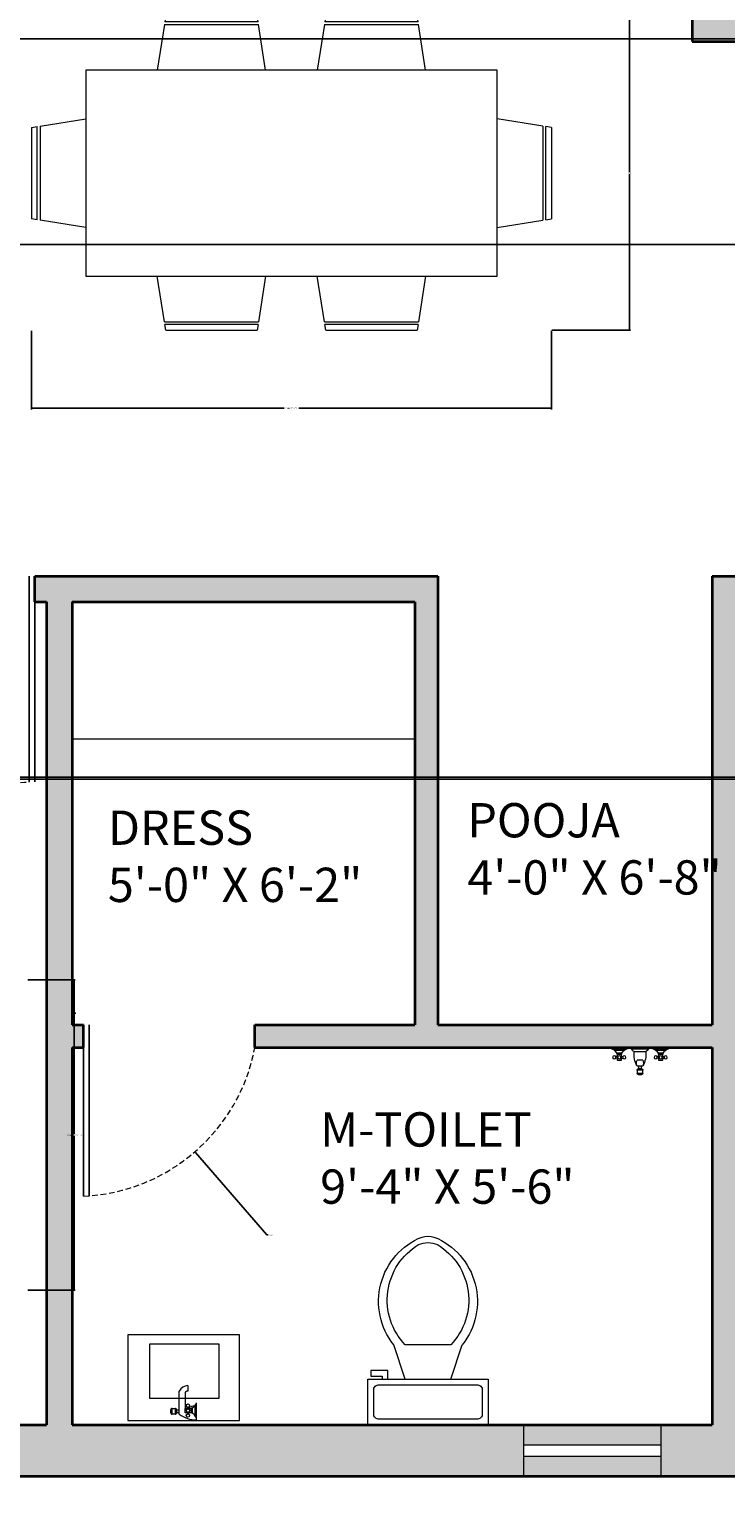
# Model space of a CAD drawing. Units: inches. Extents: x 1693 to 2974, y 2201 to 2965.
# Tile 18 of 24: x 2665 to 2787, y 2332 to 2588. Entities that reach past the tile are written whole.
import ezdxf

# ---------------------------------------------------------------- set-up
doc = ezdxf.new("R2010")
doc.units = ezdxf.units.IN
doc.header["$LTSCALE"] = 2
doc.header["$MEASUREMENT"] = 0
doc.linetypes.add('HIDDEN', pattern=[0.375, 0.25, -0.125])
for name, color, linetype, lineweight in [('A-ANNO-DIMS', 2, 'Continuous', 18), ('A-AREA-IDEN', 7, 'Continuous', 18), ('A-DOOR', 3, 'Continuous', 25), ('A-DOOR-SWNG', 3, 'HIDDEN', 13), ('A-FLOR-CASE', 32, 'Continuous', 18), ('A-FLOR-FIXT', 9, 'Continuous', 18), ('A-FURN', 8, 'Continuous', 18), ('A-GLAZ', 4, 'Continuous', 18), ('A-WALL', 7, 'Continuous', 35)]:
    doc.layers.add(name, color=color, linetype=linetype, lineweight=lineweight)
doc.layers.add('A-GLAZ-PATT', color=141, linetype='Continuous', lineweight=13, true_color=0xadddf7)
doc.layers.add('A-WALL-PATT', color=251, linetype='Continuous', lineweight=13, true_color=0x636466)
doc.styles.get("Standard").update_dxf_attribs({"font": 'arial.ttf'})
doc.dimstyles.get("Standard").update_dxf_attribs({"dimtxt": 0.18, "dimasz": 0.18, "dimexe": 0.18, "dimexo": 0.0625, "dimgap": 0.09, "dimtad": 0, "dimtih": 1, "dimtoh": 1, "dimdec": 1, "dimzin": 0, "dimdsep": 46, "dimlunit": 3, "dimtxsty": 'Standard', "dimcen": 0.09, "dimadec": 0, "dimazin": 0, "dimtfac": 1, "dimtdec": 1, "dimtofl": 0, "dimtmove": 0, "dimatfit": 3, "dimfxl": 1, "dimtolj": 1, "dimtzin": 0, "dimarcsym": 0})

# ---------------------------------------------------------------- blocks, each defined once
blk = doc.blocks.new('Toilet - top')
for p, q in [((9.5, -6), (9.5, -2)), ((-10, -8.5), (-8, -8.5)), ((-10, -9.5), (-10, -8.5)), ((-7, -9.5), (-10, -9.5)), ((-8, -8.5), (-8, -8)), ((-7, -8), (-7, -9.5)), ((-4, -8), (-6, -14)), ((4, -8), (6, -14)), ((4, -14), (-4, -14))]:
    blk.add_line(p, q)
blk.add_lwpolyline([(10.5, -8), (10.5, 0), (-10.5, 0), (-10.5, -8)], close=True)
for points in [[(-9.5, -2), (-9.5, -6)], [(8.5, -1), (-8.5, -1)], [(-8.5, -7), (8.5, -7)]]:
    blk.add_lwpolyline(points)
for centre, radius, start, end in [((-8.62, -1.88), 0.884, 81.8699, 188.1301), ((8.62, -1.88), 0.884, 351.8699, 98.1301), ((-8.62, -6.12), 0.884, 171.8699, 278.1301), ((8.62, -6.12), 0.884, 261.8699, 8.1301), ((3.52, -21.58), 12.17, 141.4691, 247.9714), ((4.2, -21.82), 11.33, 136.3677, 238.9468), ((-3.52, -21.58), 12.17, 292.0284, 38.5307), ((-4.2, -21.82), 11.33, 301.053, 43.6321), ((0, -27.88), 4, 245.7318, 294.2682), ((0, -29), 4, 254.8605, 285.1395)]:
    blk.add_arc(centre, radius, start, end)
blk = doc.blocks.new('Faucet - Bathroom side')
for p, q in [((-0.625, 4.25), (0.375, 4.25)), ((0.375, 3.75), (-0.625, 3.75)), ((-0.625, 3), (3.375, 3)), ((-0.375, 3), (-0.375, 3.5)), ((0.125, 3.5), (0.125, 3)), ((-1.625, 0), (-1.375, 0)), ((-1.375, 0), (1.375, 0)), ((-0.88366, 0.25), (0.88424, 0.25)), ((-0.375, 1.625), (-0.625, 1.625)), ((-0.375, 1.375), (-0.625, 1.375)), ((0.48078, 0.75), (-0.47286, 0.75)), ((2.875, 2), (0.375, 2)), ((0.375, 1.625), (0.625, 1.625)), ((0.375, 1.375), (0.625, 1.375)), ((4.375, 1.5), (3.375, 1.5))]:
    blk.add_line(p, q)
for points in [[(-0.625, 3.75), (-0.625, 4.25)], [(-0.375, 4.5), (0.125, 4.5)], [(0.125, 3.5), (-0.375, 3.5)], [(0.375, 4.25), (0.375, 3.75)]]:
    blk.add_lwpolyline(points)
blk.add_lwpolyline([(-0.375, 1), (-0.375, 2), (0.375, 2), (0.375, 1)], close=True)
for centre in [(-0.875, 1.5), (0, 1.5), (0.875, 1.5)]:
    blk.add_circle(centre, 0.27951)
for centre, radius, start, end in [((3.45929, -0.0281), 5.08436, 143.4467, 179.6834), ((-0.38253, 4.2575), 0.24259, 88.22243, 181.7776), ((-0.38253, 3.7424), 0.24259, 178.2224, 271.7776), ((0.13252, 4.2575), 0.24259, 358.2224, 91.77757), ((0.13252, 3.7424), 0.24259, 268.2224, 1.777565), ((2.70708, 1.4714), 1.66816, 0.9827695, 66.39737), ((-1.75, 1.375), 1.42522, 285.2551, 344.7449), ((1.75, 1.375), 1.42522, 195.2551, 254.7449), ((-2.49562, -0.286), 3.38273, 9.709485, 29.48735), ((2.96867, 1.5936), 0.41699, 347.0192, 102.9808)]:
    blk.add_arc(centre, radius, start, end)
blk = doc.blocks.new('Faucet - Bathroom front')
for p, q in [((-0.5, 4.25), (0.5, 4.25)), ((0.5, 3.75), (-0.5, 3.75)), ((-0.5, 3), (0.5, 3)), ((-0.25, 3), (-0.25, 3.5)), ((0.25, 3.5), (0.25, 3)), ((-5, 0), (-2.25, 0)), ((-4.5087, 0.25), (-2.7408, 0.25)), ((-4, 1.625), (-4.25, 1.625)), ((-4, 1.375), (-4.25, 1.375)), ((-3.1442, 0.75), (-4.0979, 0.75)), ((-3.25, 1.625), (-3, 1.625)), ((-3.25, 1.375), (-3, 1.375)), ((-1.5, 0), (1.5, 0)), ((-1, 0.5), (1, 0.5)), ((0.5, 2), (-0.5, 2)), ((2.25, 0), (5, 0)), ((2.7413, 0.25), (4.5092, 0.25)), ((3.25, 1.625), (3, 1.625)), ((3.25, 1.375), (3, 1.375)), ((4.1058, 0.75), (3.1521, 0.75)), ((4, 1.625), (4.25, 1.625)), ((4, 1.375), (4.25, 1.375))]:
    blk.add_line(p, q)
for points in [[(-0.5, 3.75), (-0.5, 4.25)], [(-0.25, 4.5), (0.25, 4.5)], [(0.25, 3.5), (-0.25, 3.5)], [(0.5, 4.25), (0.5, 3.75)]]:
    blk.add_lwpolyline(points)
for points in [[(-4, 1), (-4, 2), (-3.25, 2), (-3.25, 1)], [(3.25, 1), (3.25, 2), (4, 2), (4, 1)]]:
    blk.add_lwpolyline(points, close=True)
for centre in [(-4.5, 1.5), (-3.625, 1.5), (-2.75, 1.5), (2.75, 1.5), (3.625, 1.5), (4.5, 1.5)]:
    blk.add_circle(centre, 0.2795)
for centre, radius, start, end in [((3, 1), 4.0311, 150.2551, 187.125), ((0.6413, 2.5), 1.246, 156.3417, 203.6583), ((-0.2575, 4.2575), 0.2426, 88.22243, 181.7776), ((-0.2575, 3.7425), 0.2426, 178.2224, 271.7776), ((0.2575, 4.2575), 0.2426, 358.2224, 91.77757), ((0.2575, 3.7425), 0.2426, 268.2224, 1.777565), ((-3, 1), 4.0311, 352.875, 29.74488), ((-0.6413, 2.5), 1.246, 336.3417, 23.65835), ((-5.375, 1.375), 1.4252, 285.2551, 344.7449), ((-1.875, 1.375), 1.4252, 195.2551, 254.7449), ((-0.7962, -0.2038), 0.7327, 106.1502, 163.8498), ((0.7962, -0.2038), 0.7327, 16.1502, 73.84979), ((1.875, 1.375), 1.4252, 285.2551, 344.7449), ((5.375, 1.375), 1.4252, 195.2551, 254.7449)]:
    blk.add_arc(centre, radius, start, end)
blk = doc.blocks.new('DINING-SET-72x36-6-SEAT')
for p, q in [((23.5, 55), (23.34, 54)), ((39.66, 54), (23.35, 54)), ((23.5, 55), (39.5, 55)), ((39.66, 54), (39.5, 55)), ((51.5, 55), (51.34, 54)), ((67.66, 54), (51.35, 54)), ((51.5, 55), (67.5, 55)), ((67.66, 54), (67.5, 55)), ((23.27, 53.5), (22.02, 45.5)), ((23.27, 53.5), (39.74, 53.5)), ((40.98, 45.5), (39.73, 53.5)), ((51.27, 53.5), (50.02, 45.5)), ((51.27, 53.5), (67.74, 53.5)), ((68.98, 45.5), (67.73, 53.5)), ((81.5, 45.5), (9.5, 45.5)), ((9.5, 45.5), (9.5, 9.5)), ((81.5, 9.5), (81.5, 45.5)), ((1.5, 35.73), (9.5, 36.98)), ((89.5, 35.73), (81.5, 36.98)), ((0, 35.5), (1, 35.66)), ((0, 35.5), (0, 19.5)), ((1, 19.34), (1, 35.65)), ((1.5, 35.73), (1.5, 19.26)), ((89.5, 35.73), (89.5, 19.26)), ((91, 35.5), (90, 35.66)), ((90, 19.34), (90, 35.65)), ((91, 35.5), (91, 19.5)), ((1, 19.34), (0, 19.5)), ((9.5, 18.02), (1.5, 19.27)), ((81.5, 18.02), (89.5, 19.27)), ((90, 19.34), (91, 19.5)), ((9.5, 9.5), (81.5, 9.5)), ((23.27, 1.5), (22.02, 9.5)), ((40.98, 9.5), (39.73, 1.5)), ((51.27, 1.5), (50.02, 9.5)), ((68.98, 9.5), (67.73, 1.5)), ((23.27, 1.5), (39.74, 1.5)), ((23.5, 0), (23.34, 1)), ((39.66, 1), (23.35, 1)), ((23.5, 0), (39.5, 0)), ((39.66, 1), (39.5, 0)), ((51.27, 1.5), (67.74, 1.5)), ((51.5, 0), (51.34, 1)), ((67.66, 1), (51.35, 1)), ((51.5, 0), (67.5, 0)), ((67.66, 1), (67.5, 0))]:
    blk.add_line(p, q)
blk = doc.blocks.new('BASIN-WALL-MOUNT')
at = {"ltscale": 2}
for points in [[(15.01, 19.49), (0, 19.49), (0, 0), (15.01, 0)], [(11.1, 15.94), (1.63, 15.94), (1.63, 3.76), (11.1, 3.76)]]:
    blk.add_lwpolyline(points, close=True, dxfattribs=at)
blk = doc.blocks.new('*D47')
at = {"layer": 'A-ANNO-DIMS', "color": 0, "lineweight": -2, "ltscale": 2, "transparency": 16777216}
for p, q in [((2665.02, 2421.61), (2673.28, 2421.61)), ((2673.1, 2421.43), (2673.1, 2394.63)), ((2673.1, 2367.47), (2673.1, 2394.27)), ((2665.02, 2367.29), (2673.28, 2367.29))]:
    blk.add_line(p, q, dxfattribs=at)
at = {"layer": 'A-ANNO-DIMS', "color": 0, "ltscale": 2, "transparency": 16777216}
for points in [[(2673.07, 2421.43), (2673.13, 2421.43), (2673.1, 2421.61)], [(2673.07, 2367.47), (2673.13, 2367.47), (2673.1, 2367.29)]]:
    blk.add_solid(points, dxfattribs=at)
at = {"layer": 'Defpoints', "color": 0, "ltscale": 2, "transparency": 16777216}
for p in [(2664.96, 2421.61), (2673.1, 2421.61), (2664.96, 2367.29)]:
    blk.add_point(p, dxfattribs=at)
at = {"layer": 'A-ANNO-DIMS', "color": 0, "ltscale": 2, "transparency": 16777216, "insert": (2673.1, 2394.45), "char_height": 0.18, "attachment_point": 5}
blk.add_mtext('\\A1;TWO-SEAT SOFA 54 TYP.', dxfattribs=at)
blk = doc.blocks.new('*D61')
at = {"layer": 'A-ANNO-DIMS', "color": 0, "lineweight": -2, "ltscale": 2, "transparency": 16777216}
for p, q in [((2665.63, 2535.18), (2665.63, 2521.42)), ((2756.63, 2535.18), (2756.63, 2521.42)), ((2665.81, 2521.6), (2709.85, 2521.6)), ((2756.45, 2521.6), (2712.4, 2521.6))]:
    blk.add_line(p, q, dxfattribs=at)
at = {"layer": 'A-ANNO-DIMS', "color": 0, "ltscale": 2, "transparency": 16777216}
for points in [[(2665.81, 2521.63), (2665.81, 2521.57), (2665.63, 2521.6)], [(2756.45, 2521.63), (2756.45, 2521.57), (2756.63, 2521.6)]]:
    blk.add_solid(points, dxfattribs=at)
at = {"layer": 'Defpoints', "color": 0, "ltscale": 2, "transparency": 16777216}
for p in [(2665.63, 2535.25), (2756.63, 2535.25), (2756.63, 2521.6)]:
    blk.add_point(p, dxfattribs=at)
at = {"layer": 'A-ANNO-DIMS', "color": 0, "ltscale": 2, "transparency": 16777216, "insert": (2711.13, 2521.6), "char_height": 0.18, "attachment_point": 5}
blk.add_mtext('\\A1;DINING SET 91 TYP.', dxfattribs=at)
blk = doc.blocks.new('*D62')
at = {"layer": 'A-ANNO-DIMS', "color": 0, "lineweight": -2, "ltscale": 2, "transparency": 16777216}
for p, q in [((2756.69, 2590.25), (2770.46, 2590.25)), ((2770.28, 2590.07), (2770.28, 2562.93)), ((2770.28, 2535.43), (2770.28, 2562.56)), ((2756.69, 2535.25), (2770.46, 2535.25))]:
    blk.add_line(p, q, dxfattribs=at)
at = {"layer": 'A-ANNO-DIMS', "color": 0, "ltscale": 2, "transparency": 16777216}
for points in [[(2770.25, 2590.07), (2770.31, 2590.07), (2770.28, 2590.25)], [(2770.25, 2535.43), (2770.31, 2535.43), (2770.28, 2535.25)]]:
    blk.add_solid(points, dxfattribs=at)
at = {"layer": 'Defpoints', "color": 0, "ltscale": 2, "transparency": 16777216}
for p in [(2756.63, 2590.25), (2770.28, 2590.25), (2756.63, 2535.25)]:
    blk.add_point(p, dxfattribs=at)
at = {"layer": 'A-ANNO-DIMS', "color": 0, "ltscale": 2, "transparency": 16777216, "insert": (2770.28, 2562.75), "char_height": 0.18, "attachment_point": 5}
blk.add_mtext('\\A1;55 TYP.', dxfattribs=at)
blk = doc.blocks.new('*D81')
at = {"layer": 'A-ANNO-DIMS', "color": 0, "lineweight": -2, "ltscale": 2, "transparency": 16777216}
for p, q in [((1752.34, 2553.91), (1752.34, 2964.96)), ((1752.52, 2964.78), (2332.94, 2964.78)), ((2914.06, 2964.78), (2333.64, 2964.78)), ((2914.24, 2754.97), (2914.24, 2964.96))]:
    blk.add_line(p, q, dxfattribs=at)
at = {"layer": 'A-ANNO-DIMS', "color": 0, "ltscale": 2, "transparency": 16777216}
for points in [[(1752.52, 2964.81), (1752.52, 2964.75), (1752.34, 2964.78)], [(2914.06, 2964.81), (2914.06, 2964.75), (2914.24, 2964.78)]]:
    blk.add_solid(points, dxfattribs=at)
at = {"layer": 'Defpoints', "color": 0, "ltscale": 2, "transparency": 16777216}
for p in [(2914.24, 2964.78), (2914.24, 2754.9), (1752.34, 2553.84)]:
    blk.add_point(p, dxfattribs=at)
at = {"layer": 'A-ANNO-DIMS', "color": 0, "ltscale": 2, "transparency": 16777216, "insert": (2333.29, 2964.78), "char_height": 0.18, "attachment_point": 5}
blk.add_mtext('\\A1;1162', dxfattribs=at)
blk = doc.blocks.new('*D85')
at = {"layer": 'A-ANNO-DIMS', "color": 0, "lineweight": -2, "ltscale": 2, "transparency": 16777216}
for p, q in [((2479.24, 2334.69), (2479.24, 2200.56)), ((2902.24, 2334.69), (2902.24, 2200.56)), ((2479.42, 2200.74), (2690.44, 2200.74)), ((2902.06, 2200.74), (2691.03, 2200.74))]:
    blk.add_line(p, q, dxfattribs=at)
at = {"layer": 'A-ANNO-DIMS', "color": 0, "ltscale": 2, "transparency": 16777216}
for points in [[(2479.42, 2200.77), (2479.42, 2200.71), (2479.24, 2200.74)], [(2902.06, 2200.77), (2902.06, 2200.71), (2902.24, 2200.74)]]:
    blk.add_solid(points, dxfattribs=at)
at = {"layer": 'Defpoints', "color": 0, "ltscale": 2, "transparency": 16777216}
for p in [(2479.24, 2334.75), (2902.24, 2334.75), (2902.24, 2200.74)]:
    blk.add_point(p, dxfattribs=at)
at = {"layer": 'A-ANNO-DIMS', "color": 0, "ltscale": 2, "transparency": 16777216, "insert": (2690.74, 2200.74), "char_height": 0.18, "attachment_point": 5}
blk.add_mtext('\\A1;423', dxfattribs=at)
blk = doc.blocks.new('*D89')
at = {"layer": 'A-ANNO-DIMS', "color": 0, "lineweight": -2, "ltscale": 2, "transparency": 16777216}
for p, q in [((2479.3, 2334.75), (2973.12, 2334.75)), ((2972.94, 2334.57), (2972.94, 2312.48)), ((2972.94, 2290.02), (2972.94, 2312.12)), ((2294.3, 2289.84), (2973.12, 2289.84))]:
    blk.add_line(p, q, dxfattribs=at)
at = {"layer": 'A-ANNO-DIMS', "color": 0, "ltscale": 2, "transparency": 16777216}
for points in [[(2972.91, 2334.57), (2972.97, 2334.57), (2972.94, 2334.75)], [(2972.91, 2290.02), (2972.97, 2290.02), (2972.94, 2289.84)]]:
    blk.add_solid(points, dxfattribs=at)
at = {"layer": 'Defpoints', "color": 0, "ltscale": 2, "transparency": 16777216}
for p in [(2479.24, 2334.75), (2972.94, 2334.75), (2294.24, 2289.84)]:
    blk.add_point(p, dxfattribs=at)
at = {"layer": 'A-ANNO-DIMS', "color": 0, "ltscale": 2, "transparency": 16777216, "insert": (2972.94, 2312.3), "char_height": 0.18, "attachment_point": 5}
blk.add_mtext('\\A1;44.91', dxfattribs=at)
blk = doc.blocks.new('*D96')
at = {"layer": 'A-ANNO-DIMS', "color": 0, "lineweight": -2, "ltscale": 2, "transparency": 16777216}
for p, q in [((2294.3, 2586.26), (2973.12, 2586.26)), ((2972.94, 2586.08), (2972.94, 2568.45)), ((2972.94, 2550.44), (2972.94, 2568.08)), ((2294.3, 2550.26), (2973.12, 2550.26))]:
    blk.add_line(p, q, dxfattribs=at)
at = {"layer": 'A-ANNO-DIMS', "color": 0, "ltscale": 2, "transparency": 16777216}
for points in [[(2972.91, 2586.08), (2972.97, 2586.08), (2972.94, 2586.26)], [(2972.91, 2550.44), (2972.97, 2550.44), (2972.94, 2550.26)]]:
    blk.add_solid(points, dxfattribs=at)
at = {"layer": 'Defpoints', "color": 0, "ltscale": 2, "transparency": 16777216}
for p in [(2294.24, 2586.26), (2972.94, 2586.26), (2294.24, 2550.26)]:
    blk.add_point(p, dxfattribs=at)
at = {"layer": 'A-ANNO-DIMS', "color": 0, "ltscale": 2, "transparency": 16777216, "insert": (2972.94, 2568.26), "char_height": 0.18, "attachment_point": 5}
blk.add_mtext('\\A1;36', dxfattribs=at)
blk = doc.blocks.new('*D97')
at = {"layer": 'A-ANNO-DIMS', "color": 0, "lineweight": -2, "ltscale": 2, "transparency": 16777216}
for p, q in [((2294.3, 2631.75), (2973.12, 2631.75)), ((2972.94, 2631.57), (2972.94, 2609.19)), ((2972.94, 2586.44), (2972.94, 2608.83)), ((2294.3, 2586.26), (2973.12, 2586.26))]:
    blk.add_line(p, q, dxfattribs=at)
at = {"layer": 'A-ANNO-DIMS', "color": 0, "ltscale": 2, "transparency": 16777216}
for points in [[(2972.91, 2631.57), (2972.97, 2631.57), (2972.94, 2631.75)], [(2972.91, 2586.44), (2972.97, 2586.44), (2972.94, 2586.26)]]:
    blk.add_solid(points, dxfattribs=at)
at = {"layer": 'Defpoints', "color": 0, "ltscale": 2, "transparency": 16777216}
for p in [(2294.24, 2631.75), (2972.94, 2631.75), (2294.24, 2586.26)]:
    blk.add_point(p, dxfattribs=at)
at = {"layer": 'A-ANNO-DIMS', "color": 0, "ltscale": 2, "transparency": 16777216, "insert": (2972.94, 2609.01), "char_height": 0.18, "attachment_point": 5}
blk.add_mtext('\\A1;45.49', dxfattribs=at)
blk = doc.blocks.new('*D108')
at = {"layer": 'A-ANNO-DIMS', "color": 0, "lineweight": -2, "ltscale": 2, "transparency": 16777216}
for p, q in [((2972.94, 2457.27), (2972.94, 2457.45)), ((2972.94, 2457.45), (2973.12, 2457.45)), ((1752.74, 2457.09), (2973.12, 2457.09)), ((1752.74, 2456.73), (2973.12, 2456.73)), ((2972.94, 2456.55), (2972.94, 2456.37))]:
    blk.add_line(p, q, dxfattribs=at)
at = {"layer": 'A-ANNO-DIMS', "color": 0, "ltscale": 2, "transparency": 16777216}
for points in [[(2972.91, 2457.27), (2972.97, 2457.27), (2972.94, 2457.09)], [(2972.91, 2456.55), (2972.97, 2456.55), (2972.94, 2456.73)]]:
    blk.add_solid(points, dxfattribs=at)
at = {"layer": 'Defpoints', "color": 0, "ltscale": 2, "transparency": 16777216}
for p in [(1752.68, 2457.09), (1752.68, 2456.73), (2972.94, 2457.09)]:
    blk.add_point(p, dxfattribs=at)
at = {"layer": 'A-ANNO-DIMS', "color": 0, "ltscale": 2, "transparency": 16777216, "insert": (2973.44, 2457.45), "char_height": 0.18, "attachment_point": 5}
blk.add_mtext('\\A1;0.36', dxfattribs=at)
blk = doc.blocks.new('*D117')
at = {"layer": 'A-ANNO-DIMS', "color": 0, "lineweight": -2, "ltscale": 2, "transparency": 16777216}
for p, q in [((2673.17, 2415.77), (2673.35, 2415.77)), ((2673.26, 2415.68), (2673.26, 2415.86)), ((2706.84, 2377.02), (2694.36, 2391.41)), ((2707.02, 2377.02), (2706.84, 2377.02))]:
    blk.add_line(p, q, dxfattribs=at)
at = {"layer": 'A-ANNO-DIMS', "color": 0, "ltscale": 2, "transparency": 16777216}
blk.add_solid([(2694.39, 2391.43), (2694.34, 2391.39), (2694.25, 2391.55)], dxfattribs=at)
at = {"layer": 'Defpoints', "color": 0, "ltscale": 2, "transparency": 16777216}
for p in [(2673.26, 2415.77), (2694.25, 2391.55)]:
    blk.add_point(p, dxfattribs=at)
at = {"layer": 'A-ANNO-DIMS', "color": 0, "ltscale": 2, "transparency": 16777216, "insert": (2707.5, 2377.02), "char_height": 0.18, "attachment_point": 5}
blk.add_mtext('\\A1;R32.05', dxfattribs=at)

msp = doc.modelspace()

# ---------------------------------------------------------------- hatches: boundary and pattern name
at = {"layer": 'A-GLAZ-PATT', "ltscale": 2}
h = msp.add_hatch(color=256, dxfattribs=at)
h.dxf.hatch_style = 1
h.paths.add_polyline_path([(2656.9702, 2338.2547), (2632.9702, 2338.2547), (2632.9702, 2339.2547), (2608.9702, 2339.2547), (2608.9702, 2334.7547), (2656.9702, 2334.7547)])
h.paths.add_polyline_path([(2656.9702, 2343.7547), (2608.9702, 2343.7547), (2608.9702, 2340.2547), (2632.9702, 2340.2547), (2632.9702, 2339.2547), (2656.9702, 2339.2547)])
h.paths.add_polyline_path([(2775.7544, 2338.2547), (2751.7544, 2338.2547), (2751.7544, 2334.7547), (2775.7544, 2334.7547)])
h.paths.add_polyline_path([(2775.7544, 2343.7547), (2751.7544, 2343.7547), (2751.7544, 2340.2547), (2775.7544, 2340.2547)])
h.paths.add_polyline_path([(2897.7363, 2568.7999), (2893.2363, 2568.7999), (2893.2363, 2520.7999), (2896.7363, 2520.7999), (2896.7363, 2544.7999), (2897.7363, 2544.7999)])
h.paths.add_polyline_path([(2902.2363, 2568.7999), (2898.7363, 2568.7999), (2898.7363, 2544.7999), (2897.7363, 2544.7999), (2897.7363, 2520.7999), (2902.2363, 2520.7999)])
h.paths.add_polyline_path([(2902.2363, 2637.7547), (2898.7363, 2637.7547), (2898.7363, 2613.7547), (2902.2363, 2613.7547)])
h.paths.add_polyline_path([(2896.7363, 2637.7547), (2893.2363, 2637.7547), (2893.2363, 2613.7547), (2896.7363, 2613.7547)])
h.paths.add_polyline_path([(2902.2363, 2748.903), (2899.0477, 2748.903), (2899.0477, 2724.903), (2898.0477, 2724.903), (2898.0477, 2700.903), (2902.2363, 2700.903)])
h.paths.add_polyline_path([(2898.0477, 2748.903), (2893.2363, 2748.903), (2893.2363, 2700.903), (2897.0477, 2700.903), (2897.0477, 2724.903), (2898.0477, 2724.903)])
h.paths.add_polyline_path([(2851.2363, 2846.2547), (2803.2363, 2846.2547), (2803.2363, 2842.7547), (2827.2363, 2842.7547), (2827.2363, 2841.7547), (2851.2363, 2841.7547)])
h.paths.add_polyline_path([(2851.2363, 2840.7547), (2827.2363, 2840.7547), (2827.2363, 2841.7547), (2803.2363, 2841.7547), (2803.2363, 2837.2547), (2851.2363, 2837.2547)])
h.paths.add_polyline_path([(2578.2363, 2846.2547), (2530.2363, 2846.2547), (2530.2363, 2842.7547), (2554.2363, 2842.7547), (2554.2363, 2841.7547), (2578.2363, 2841.7547)])
h.paths.add_polyline_path([(2578.2363, 2840.7547), (2554.2363, 2840.7547), (2554.2363, 2841.7547), (2530.2363, 2841.7547), (2530.2363, 2837.2547), (2578.2363, 2837.2547)])
h.paths.add_polyline_path([(2732.7363, 2812.7547), (2705.1363, 2812.7547), (2705.1363, 2811.7547), (2676.3363, 2811.7547), (2676.3363, 2812.7547), (2648.7363, 2812.7547), (2648.7363, 2808.2547), (2732.7363, 2808.2547)])
h.paths.add_polyline_path([(2732.7363, 2817.2547), (2648.7363, 2817.2547), (2648.7363, 2813.7547), (2676.3363, 2813.7547), (2676.3363, 2812.7547), (2705.1363, 2812.7547), (2705.1363, 2813.7547), (2732.7363, 2813.7547)])
h.paths.add_polyline_path([(2488.2363, 2695.8203), (2484.7878, 2695.8203), (2484.7878, 2671.8203), (2488.2363, 2671.8203)])
h.paths.add_polyline_path([(2482.7878, 2695.8203), (2479.2363, 2695.8203), (2479.2363, 2671.8203), (2482.7878, 2671.8203)])
h.paths.add_polyline_path([(2488.2363, 2572.4371), (2484.7363, 2572.4371), (2484.7363, 2541.4371), (2483.7363, 2541.4371), (2483.7363, 2512.4371), (2488.2363, 2512.4371)])
h.paths.add_polyline_path([(2482.7363, 2541.4371), (2483.7363, 2541.4371), (2483.7363, 2572.4371), (2479.2363, 2572.4371), (2479.2363, 2512.4371), (2482.7363, 2512.4371)])
h.paths.add_polyline_path([(2248.9863, 2706.8449), (2190.9863, 2706.8449), (2190.9863, 2703.3449), (2219.9863, 2703.3449), (2219.9863, 2702.3449), (2248.9863, 2702.3449)])
h.paths.add_polyline_path([(2248.9863, 2701.3449), (2219.9863, 2701.3449), (2219.9863, 2702.3449), (2190.9863, 2702.3449), (2190.9863, 2697.8449), (2248.9863, 2697.8449)])
h.paths.add_polyline_path([(2151.9207, 2293.3449), (2127.9207, 2293.3449), (2127.9207, 2289.8449), (2151.9207, 2289.8449)])
h.paths.add_polyline_path([(2151.9207, 2298.8449), (2127.9207, 2298.8449), (2127.9207, 2295.3449), (2151.9207, 2295.3449)])
h.paths.add_polyline_path([(2084.023, 2293.3449), (2066.023, 2293.3449), (2066.023, 2294.3449), (2048.023, 2294.3449), (2048.023, 2289.8449), (2084.023, 2289.8449)])
h.paths.add_polyline_path([(2084.023, 2298.8449), (2048.023, 2298.8449), (2048.023, 2295.3449), (2066.023, 2295.3449), (2066.023, 2294.3449), (2084.023, 2294.3449)])
h.paths.add_polyline_path([(1966.0781, 2293.3449), (1948.0781, 2293.3449), (1948.0781, 2294.3449), (1930.0781, 2294.3449), (1930.0781, 2289.8449), (1966.0781, 2289.8449)])
h.paths.add_polyline_path([(1966.0781, 2298.8449), (1930.0781, 2298.8449), (1930.0781, 2295.3449), (1948.0781, 2295.3449), (1948.0781, 2294.3449), (1966.0781, 2294.3449)])
h.paths.add_polyline_path([(1787.2363, 2403.1922), (1782.7363, 2403.1922), (1782.7363, 2355.1922), (1786.2363, 2355.1922), (1786.2363, 2379.1922), (1787.2363, 2379.1922)])
h.paths.add_polyline_path([(1791.7363, 2403.1922), (1788.2363, 2403.1922), (1788.2363, 2379.1922), (1787.2363, 2379.1922), (1787.2363, 2355.1922), (1791.7363, 2355.1922)])
h.paths.add_polyline_path([(1786.2363, 2477.5455), (1782.7363, 2477.5455), (1782.7363, 2453.5455), (1786.2363, 2453.5455)])
h.paths.add_polyline_path([(1791.7363, 2477.5455), (1788.2363, 2477.5455), (1788.2363, 2453.5455), (1791.7363, 2453.5455)])
h.paths.add_polyline_path([(1786.2363, 2621.6433), (1782.7363, 2621.6433), (1782.7363, 2585.6433), (1786.2363, 2585.6433)])
h.paths.add_polyline_path([(1791.7363, 2621.6433), (1788.2363, 2621.6433), (1788.2363, 2585.6433), (1791.7363, 2585.6433)])
h.paths.add_polyline_path([(1908.1286, 2706.8449), (1860.1286, 2706.8449), (1860.1286, 2703.3449), (1884.1286, 2703.3449), (1884.1286, 2702.3449), (1908.1286, 2702.3449)])
h.paths.add_polyline_path([(1908.1286, 2701.3449), (1884.1286, 2701.3449), (1884.1286, 2702.3449), (1860.1286, 2702.3449), (1860.1286, 2697.8449), (1908.1286, 2697.8449)])
h.paths.add_polyline_path([(1973.9863, 2706.8449), (1949.9863, 2706.8449), (1949.9863, 2703.3449), (1973.9863, 2703.3449)])
h.paths.add_polyline_path([(1973.9863, 2701.3449), (1949.9863, 2701.3449), (1949.9863, 2697.8449), (1973.9863, 2697.8449)])
h.paths.add_polyline_path([(2112.7363, 2690.3449), (2028.7363, 2690.3449), (2028.7363, 2686.8449), (2056.3363, 2686.8449), (2056.3363, 2685.8449), (2085.1363, 2685.8449), (2085.1363, 2686.8449), (2112.7363, 2686.8449)])
h.paths.add_polyline_path([(2112.7363, 2685.8449), (2085.1363, 2685.8449), (2085.1363, 2684.8449), (2056.3363, 2684.8449), (2056.3363, 2685.8449), (2028.7363, 2685.8449), (2028.7363, 2681.3449), (2112.7363, 2681.3449)])
h.paths.add_polyline_path([(2422.7363, 2640.7547), (2350.7363, 2640.7547), (2350.7363, 2637.2547), (2386.7363, 2637.2547), (2386.7363, 2636.2547), (2422.7363, 2636.2547)])
h.paths.add_polyline_path([(2422.7363, 2635.2547), (2386.7363, 2635.2547), (2386.7363, 2636.2547), (2350.7363, 2636.2547), (2350.7363, 2631.7547), (2422.7363, 2631.7547)])
at = {"layer": 'A-WALL-PATT', "ltscale": 2}
h = msp.add_hatch(color=256, dxfattribs=at)
h.dxf.hatch_style = 1
h.paths.add_polyline_path([(1928.2363, 2733.2161), (1930.9384, 2733.2161), (1930.9384, 2737.2161), (1923.7363, 2737.2161), (1923.7363, 2706.8449), (1908.1286, 2706.8449), (1908.1286, 2697.8449), (1923.7363, 2697.8449), (1923.7363, 2692.8449), (1928.2363, 2692.8449), (1928.2363, 2697.8449), (1949.9863, 2697.8449), (1949.9863, 2706.8449), (1928.2363, 2706.8449)])
h.paths.add_polyline_path([(2004.7363, 2737.2161), (1995.7363, 2737.2161), (1995.7363, 2706.8449), (1985.6374, 2706.8449), (1973.9863, 2706.8449), (1973.9863, 2697.8449), (2000.2363, 2697.8449), (2000.2363, 2686.5348), (2000.3613, 2686.5348), (2000.3613, 2667.0432), (2000.2363, 2601.8449), (1928.2363, 2601.8449), (1928.2363, 2662.8449), (1923.7363, 2662.8449), (1923.7363, 2595.3449), (1928.2363, 2595.3449), (1928.2363, 2597.3449), (2004.7363, 2597.3449), (2004.7363, 2681.3449), (2012.7814, 2681.3449), (2028.7363, 2681.3449), (2028.7363, 2690.3449), (2004.7363, 2690.3449)])
h.paths.add_polyline_path([(2190.9863, 2706.8449), (2184.9863, 2706.8449), (2145.7363, 2706.8449), (2145.7363, 2765.3449), (2145.7363, 2774.5394), (2136.7363, 2774.5394), (2136.7363, 2756.3449), (2136.7363, 2690.3449), (2112.7363, 2690.3449), (2112.7363, 2681.3449), (2136.7363, 2681.3449), (2136.7363, 2597.3449), (2141.2363, 2597.3449), (2141.2363, 2697.8449), (2190.9863, 2697.8449)])
h.paths.add_polyline_path([(1860.1286, 2706.8449), (1782.7363, 2706.8449), (1782.7363, 2621.6433), (1791.7363, 2621.6433), (1791.7363, 2697.8449), (1860.1286, 2697.8449)])
h.paths.add_polyline_path([(1791.7363, 2585.6433), (1782.7363, 2585.6433), (1782.7363, 2562.8449), (1782.7363, 2553.8449), (1752.3363, 2553.8449), (1752.3363, 2544.2586), (1756.3363, 2544.2586), (1756.3363, 2549.3449), (1782.7363, 2549.3449), (1782.7363, 2489.2404), (1782.7363, 2477.5455), (1791.7363, 2477.5455), (1791.7363, 2493.5991), (1791.6113, 2493.5991), (1791.6113, 2513.0907), (1791.6824, 2533.7198, -0.94742783), (1791.7363, 2534.7168), (1791.7363, 2549.3449), (1863.7363, 2549.3449), (1863.7363, 2513.3449), (1866.7363, 2513.3449), (1866.7363, 2549.3449), (1924.7363, 2549.3449), (1924.7363, 2447.3449), (1924.7363, 2442.8449), (1933.7363, 2442.8449), (1933.7363, 2447.3449), (1928.2363, 2447.3449), (1928.2363, 2559.3449), (1923.7363, 2559.3449), (1923.7363, 2553.8449), (1791.7363, 2553.8449), (1791.7363, 2562.8449)])
h.paths.add_polyline_path([(1791.7363, 2442.8449), (1866.7363, 2442.8449), (1866.7363, 2447.3449), (1866.7363, 2483.3449), (1863.7363, 2483.3449), (1863.7363, 2447.3449), (1791.7363, 2447.3449), (1791.7363, 2453.5455), (1782.7363, 2453.5455), (1782.7363, 2447.3449), (1756.3363, 2447.3449), (1756.3363, 2455.7126), (1752.3363, 2455.7126), (1752.3363, 2442.8449), (1782.7363, 2442.8449), (1782.7363, 2403.1922), (1791.7363, 2403.1922)])
h.paths.add_polyline_path([(1930.0781, 2298.8449), (1791.7363, 2298.8449), (1791.7363, 2355.1922), (1782.7363, 2355.1922), (1782.7363, 2289.8449), (1930.0781, 2289.8449)])
h.paths.add_polyline_path([(2624.7363, 2883.2547), (2624.7363, 2902.6165), (2624.7363, 2906.0761), (2615.7363, 2906.0761), (2615.7363, 2892.2547), (2615.7363, 2846.2547), (2578.2363, 2846.2547), (2578.2363, 2837.2547), (2620.2363, 2837.2547), (2620.2363, 2743.2547), (2624.7363, 2743.2547), (2624.7363, 2808.2547), (2648.7363, 2808.2547), (2648.7363, 2817.2547), (2624.7363, 2817.2547)])
h.paths.add_polyline_path([(2530.2363, 2846.2547), (2479.2363, 2846.2547), (2479.2363, 2695.8203), (2488.2363, 2695.8203), (2488.2363, 2700.7547), (2567.2363, 2700.7547), (2567.2363, 2705.2547), (2488.2363, 2705.2547), (2488.2363, 2837.2547), (2530.2363, 2837.2547)])
h.paths.add_polyline_path([(2488.2363, 2487.7547), (2630.2363, 2487.7547, -0.00990191), (2630.2363, 2489.0322), (2630.2363, 2492.2547), (2488.2363, 2492.2547), (2488.2363, 2512.4371), (2479.2363, 2512.4371), (2479.2363, 2334.7547), (2608.9702, 2334.7547), (2608.9702, 2343.7547), (2488.2363, 2343.7547)])
h.paths.add_polyline_path([(2751.7544, 2343.7547), (2672.7363, 2343.7547), (2672.7363, 2409.7547), (2674.7363, 2409.7547), (2674.7363, 2413.7547), (2672.7363, 2413.7547), (2672.7363, 2487.7547), (2732.7363, 2487.7547), (2732.7363, 2413.7547), (2704.7363, 2413.7547), (2704.7363, 2409.7547), (2784.7363, 2409.7547), (2784.7363, 2343.7547), (2775.7544, 2343.7547), (2775.7544, 2334.7547), (2902.2363, 2334.7547), (2902.2363, 2520.7999), (2893.2363, 2520.7999), (2893.2363, 2413.7547), (2856.0145, 2413.7547), (2856.0145, 2409.7547), (2893.2363, 2409.7547), (2893.2363, 2343.7547), (2789.2363, 2343.7547), (2789.2363, 2409.7547), (2819.2363, 2409.7547), (2826.0145, 2409.7547), (2826.0145, 2413.7547), (2789.2363, 2413.7547), (2789.2363, 2492.2547), (2784.7363, 2492.2547), (2784.7363, 2413.7547), (2736.7363, 2413.7547), (2736.7363, 2492.2547), (2672.7363, 2492.2547), (2666.2363, 2492.2547), (2666.2363, 2487.7547), (2668.2363, 2487.7547), (2668.2363, 2343.7547), (2656.9702, 2343.7547), (2656.9702, 2334.7547), (2662.9702, 2334.7547), (2751.7544, 2334.7547)])
h.paths.add_polyline_path([(2902.2363, 2613.7547), (2893.2363, 2613.7547), (2893.2363, 2589.7547), (2785.2363, 2589.7547), (2785.2363, 2661.7547), (2790.2363, 2661.7547), (2790.2363, 2665.2547), (2761.2363, 2665.2547), (2761.2363, 2667.2547), (2756.7363, 2667.2547), (2756.7363, 2661.7547), (2781.2363, 2661.7547), (2781.2363, 2585.7547), (2893.2363, 2585.7547), (2893.2363, 2568.7999), (2902.2363, 2568.7999)])
h.paths.add_polyline_path([(2488.2363, 2671.8203), (2479.2363, 2671.8203), (2479.2363, 2645.2547), (2479.2363, 2623.4598), (2488.2363, 2623.4598), (2488.2363, 2636.2547), (2624.7363, 2636.2547), (2624.7363, 2640.7547), (2603.7363, 2640.7547), (2603.7363, 2700.7547), (2624.7363, 2700.7547), (2624.7363, 2707.2547), (2620.2363, 2707.2547), (2620.2363, 2705.2547), (2597.2363, 2705.2547), (2597.2363, 2700.7547), (2599.2363, 2700.7547), (2599.2363, 2640.7547), (2488.2363, 2640.7547)])
h.paths.add_polyline_path([(2761.2363, 2837.2547), (2803.2363, 2837.2547), (2803.2363, 2846.2547), (2797.2363, 2846.2547), (2765.7363, 2846.2547), (2756.7363, 2846.2547), (2756.7363, 2817.2547), (2732.7363, 2817.2547), (2732.7363, 2808.2547), (2756.7363, 2808.2547), (2756.7363, 2703.2547), (2761.2363, 2703.2547)])
h.paths.add_polyline_path([(2739.7489, 2433.1234), (2786.9181, 2433.1234), (2786.9181, 2455.5122), (2739.7489, 2455.5122)], flags=25)

# ---------------------------------------------------------------- linework, layer by layer
at = {"layer": 'A-DOOR', "ltscale": 2}
for p, q in [((2665.2363, 2492.2547), (2665.2363, 2456.2547)), ((2666.2363, 2492.2547), (2666.2363, 2456.2547)), ((2674.7363, 2413.7547), (2674.7363, 2383.7547)), ((2675.7363, 2413.7547), (2675.7363, 2383.7547))]:
    msp.add_line(p, q, dxfattribs=at)
at = {"layer": 'A-DOOR-SWNG', "ltscale": 2}
for centre, radius, start, end in [((2662.4862, 2488.3934), 32.2562, 178.865361, 274.890936), ((2673.2558, 2415.7707), 32.0502, 272.647654, 349.181112)]:
    msp.add_arc(centre, radius, start, end, dxfattribs=at)
at = {"layer": 'A-FLOR-CASE', "ltscale": 2}
msp.add_line((2672.7363, 2463.7547), (2732.7363, 2463.7547), dxfattribs=at)
at = {"layer": 'A-GLAZ', "ltscale": 2}
for p, q in [((2751.7544, 2343.7547), (2751.7544, 2334.7547)), ((2775.7544, 2343.7547), (2775.7544, 2334.7547)), ((2751.7544, 2340.2547), (2775.7544, 2340.2547)), ((2751.7544, 2338.2547), (2775.7544, 2338.2547))]:
    msp.add_line(p, q, dxfattribs=at)
at = {"layer": 'A-WALL'}
for p, q in [((2781.2363, 2661.7547), (2781.2363, 2585.7547)), ((2736.7363, 2492.2547), (2736.7363, 2413.7547)), ((2784.7363, 2492.2547), (2784.7363, 2413.7547)), ((2668.2363, 2487.7547), (2668.2363, 2343.7547)), ((2672.7363, 2487.7547), (2672.7363, 2413.7547)), ((2732.7363, 2487.7547), (2732.7363, 2413.7547)), ((2672.7363, 2409.7547), (2672.7363, 2343.7547)), ((2784.7363, 2409.7547), (2784.7363, 2343.7547))]:
    msp.add_line(p, q, dxfattribs=at)
at = {"layer": 'A-WALL', "ltscale": 2}
for p, q in [((2781.2363, 2585.7547), (2893.2363, 2585.7547)), ((2666.2363, 2487.7547), (2666.2363, 2492.2547)), ((2666.2363, 2492.2547), (2672.7363, 2492.2547)), ((2672.7363, 2492.2547), (2736.7363, 2492.2547)), ((2784.7363, 2492.2547), (2789.2363, 2492.2547)), ((2666.2363, 2487.7547), (2668.2363, 2487.7547)), ((2672.7363, 2487.7547), (2732.7363, 2487.7547)), ((2672.7363, 2413.7547), (2674.7363, 2413.7547)), ((2674.7363, 2409.7547), (2674.7363, 2413.7547)), ((2704.7363, 2409.7547), (2704.7363, 2413.7547)), ((2704.7363, 2413.7547), (2732.7363, 2413.7547)), ((2736.7363, 2413.7547), (2784.7363, 2413.7547)), ((2672.7363, 2409.7547), (2674.7363, 2409.7547)), ((2704.7363, 2409.7547), (2784.7363, 2409.7547)), ((2488.2363, 2343.7547), (2668.2363, 2343.7547)), ((2672.7363, 2343.7547), (2784.7363, 2343.7547)), ((2479.2363, 2334.7547), (2902.2363, 2334.7547))]:
    msp.add_line(p, q, dxfattribs=at)

# ---------------------------------------------------------------- block references
at = {"layer": 'A-FLOR-FIXT', "ltscale": 2, "xscale": -1, "rotation": 180}
for name, p in [('Faucet - Bathroom front', (2772.1042, 2409.5509)), ('Toilet - top', (2735.0154, 2343.7547))]:
    msp.add_blockref(name, p, dxfattribs=at)
at = {"layer": 'A-FLOR-FIXT', "rotation": 270.0000000000056}
msp.add_blockref('BASIN-WALL-MOUNT', (2682.5159, 2359.5136), dxfattribs=at)
at = {"layer": 'A-FLOR-FIXT', "ltscale": 2, "rotation": 89.99999999999996}
msp.add_blockref('Faucet - Bathroom side', (2694.4967, 2346.2503), dxfattribs=at)
at = {"layer": 'A-FURN'}
msp.add_blockref('DINING-SET-72x36-6-SEAT', (2665.6267, 2535.2453), dxfattribs=at)

# ---------------------------------------------------------------- texts
at = {"layer": 'A-AREA-IDEN', "ltscale": 2, "char_height": 6, "attachment_point": 1}
for s, insert in [('POOJA \\P4\'-0" X 6\'-8"', (2741.8956, 2452.5307)), ('DRESS\\P5\'-0" X 6\'-2"', (2678.9907, 2451.228)), ('M-TOILET\\P9\'-4" X 5\'-6"', (2716.1426, 2398.4368))]:
    msp.add_mtext_dynamic_manual_height_columns(s, width=108.452746, gutter_width=1, heights=[0], dxfattribs=dict(at, insert=insert))

# ---------------------------------------------------------------- dimensions: what is measured, and where the dimension line sits
at = {"layer": 'A-ANNO-DIMS', "ltscale": 2}
for base, p1, p2, picture, middle in [((2914.2363, 2964.7761), (1752.3363, 2553.8449), (2914.2363, 2754.903), '*D81', (2333.2863, 2964.7761)), ((2902.2363, 2200.7449), (2479.2363, 2334.7547), (2902.2363, 2334.7547), '*D85', (2690.7363, 2200.7449))]:
    dim = msp.add_linear_dim(base=base, p1=p1, p2=p2, dimstyle='Standard', override={"dimdec": 0, "dimlfac": 1, "dimrnd": 0, "dimzin": 0, "dimdsep": 46, "dimlunit": 2}, dxfattribs=at)
    dim.commit()
    dim.dimension.update_dxf_attribs({"geometry": picture, "text_midpoint": middle})
for base, p1, p2, override, picture, middle in [((2972.9363, 2631.7547), (2294.2363, 2586.2648), (2294.2363, 2631.7547), {"dimdec": 2, "dimlfac": 1, "dimrnd": 0, "dimzin": 0, "dimdsep": 46, "dimlunit": 2}, '*D97', (2972.9363, 2609.0097)), ((2972.9363, 2586.2648), (2294.2363, 2550.2648), (2294.2363, 2586.2648), {"dimdec": 0, "dimlfac": 1, "dimrnd": 0, "dimzin": 0, "dimdsep": 46, "dimlunit": 2}, '*D96', (2972.9363, 2568.2648)), ((2972.9363, 2457.0877), (1752.6754, 2456.7302), (1752.6754, 2457.0877), {"dimdec": 2, "dimlfac": 1, "dimrnd": 0, "dimzin": 0, "dimdsep": 46, "dimlunit": 2}, '*D108', (2973.44, 2457.4477)), ((2972.9363, 2334.7547), (2294.2363, 2289.8449), (2479.2363, 2334.7547), {"dimdec": 2, "dimlfac": 1, "dimrnd": 0, "dimzin": 0, "dimdsep": 46, "dimlunit": 2}, '*D89', (2972.9363, 2312.2998))]:
    dim = msp.add_linear_dim(base=base, p1=p1, p2=p2, angle=90, dimstyle='Standard', override=override, dxfattribs=at)
    dim.commit()
    dim.dimension.update_dxf_attribs({"geometry": picture, "text_midpoint": middle})
for base, p1, p2, text, picture, middle in [((2770.2768, 2590.2455), (2756.6268, 2535.2455), (2756.6268, 2590.2455), '<> TYP.', '*D62', (2770.2768, 2562.7455)), ((2673.1032, 2421.6075), (2664.9563, 2367.2948), (2664.9563, 2421.6075), 'TWO-SEAT SOFA <> TYP.', '*D47', (2673.1032, 2394.4511))]:
    dim = msp.add_linear_dim(base=base, p1=p1, p2=p2, angle=90, text=text, dimstyle='Standard', override={"dimdec": 0, "dimlfac": 1, "dimrnd": 0, "dimzin": 0, "dimdsep": 46, "dimlunit": 2}, dxfattribs=at)
    dim.commit()
    dim.dimension.update_dxf_attribs({"geometry": picture, "text_midpoint": middle})
dim = msp.add_linear_dim(base=(2756.6268, 2521.5955), p1=(2665.6268, 2535.2455), p2=(2756.6268, 2535.2455), text='DINING SET <> TYP.', dimstyle='Standard', override={"dimdec": 0, "dimlfac": 1, "dimrnd": 0, "dimzin": 0, "dimdsep": 46, "dimlunit": 2}, dxfattribs=at)
dim.commit()
dim.dimension.update_dxf_attribs({"geometry": '*D61', "text_midpoint": (2711.1268, 2521.5955)})
dim = msp.add_radius_dim(center=(2673.2558, 2415.7707), mpoint=(2694.2463, 2391.5506), dimstyle='Standard', override={"dimdec": 2, "dimlfac": 1, "dimrnd": 0, "dimzin": 0, "dimdsep": 46, "dimlunit": 2}, dxfattribs=at)
dim.commit()
dim.dimension.update_dxf_attribs({"geometry": '*D117', "text_midpoint": (2707.5012, 2377.0186), "dimtype": 164})

doc.saveas('drawing.dxf')
